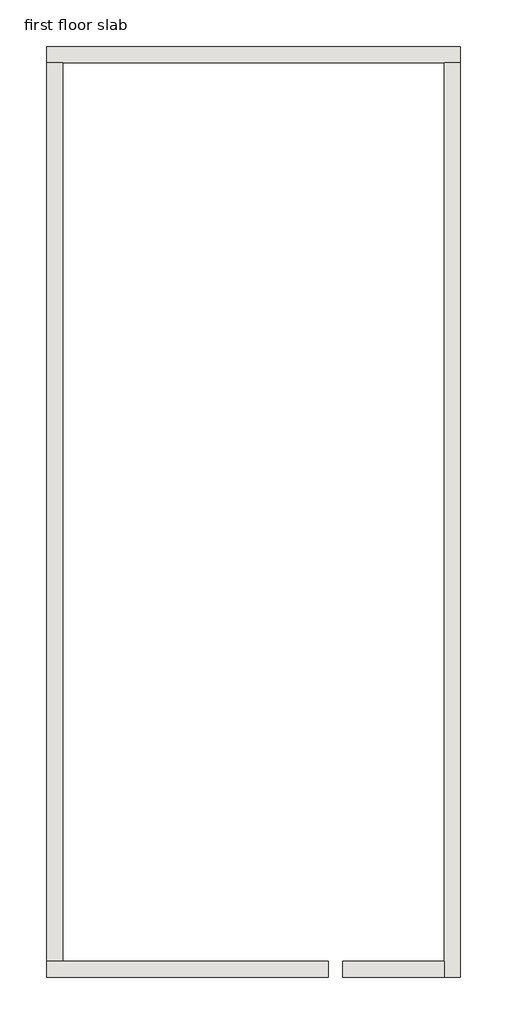
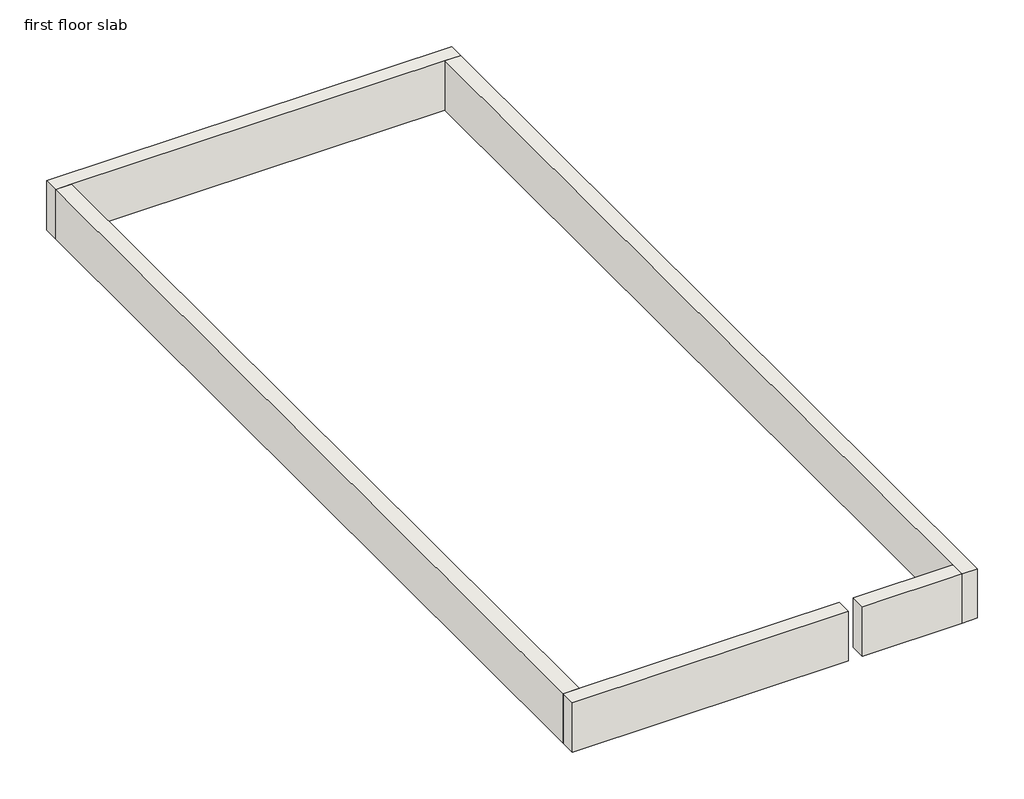
# One storey: 5 walls.
"""IFC4 building model written with IfcOpenShell, lengths in millimetres."""

from ifc_helpers import new_model, si_unit, frame, origin, place, context, project, spatial, polyline, outline, extrude, faceted_brep, element, save

model = new_model("IFC4")

# Units and contexts
model_context = context("Model", 3, world=origin())
ifc_project = project(units=[si_unit("LENGTHUNIT", "METRE", prefix="MILLI")], contexts=[model_context])

# Site, building, storey
site = spatial("IfcSite", under=ifc_project)
building = spatial("IfcBuilding", under=site)
storey = spatial("IfcBuildingStorey", under=building, Name="first floor slab", Elevation=6705.6)

# Walls
placement = place(None, origin())
element("IfcWall", 1, ObjectType="wall 9\"", at=placement, inside=storey, context=model_context, shape_type="Brep", body=[
    faceted_brep([(-12403.8986863, -3151.661407, 6705.6), (-16197.9371373, -3151.661407, 6705.6), (-16426.5371373, -3151.661407, 6705.6), (-16426.5371373, -3151.661407, 7467.6), (-16197.9371373, -3151.661407, 7467.6), (-12403.8986863, -3151.661407, 7467.6), (-12403.8986863, -3380.261407, 6705.6), (-12403.8986863, -3380.261407, 7467.6), (-16426.5371373, -3380.261407, 7467.6), (-16426.5371373, -3380.261407, 6705.6)], [[[0, 1, 2, 3, 4, 5]], [[6, 7, 8, 9]], [[2, 1, 0, 6, 9]], [[5, 4, 3, 8, 7]], [[0, 5, 7, 6]], [[3, 2, 9, 8]]]),
])
element("IfcWall", 2, ObjectType="wall 9\"", at=placement, inside=storey, context=model_context, shape_type="Brep", body=[
    faceted_brep([(-16426.5371373, 9675.338593, 6705.6), (-16197.9371373, 9675.338593, 6705.6), (-10749.6371373, 9675.338593, 6705.6), (-10521.0371373, 9675.338593, 6705.6), (-10521.0371373, 9675.338593, 7467.6), (-10749.6371373, 9675.338593, 7467.6), (-16197.9371373, 9675.338593, 7467.6), (-16426.5371373, 9675.338593, 7467.6), (-16426.5371373, 9903.938593, 6705.6), (-16426.5371373, 9903.938593, 7467.6), (-10521.0371373, 9903.938593, 7467.6), (-10521.0371373, 9903.938593, 6705.6)], [[[0, 1, 2, 3, 4, 5, 6, 7]], [[8, 9, 10, 11]], [[3, 2, 1, 0, 8, 11]], [[7, 6, 5, 4, 10, 9]], [[4, 3, 11, 10]], [[0, 7, 9, 8]]]),
])
element("IfcWall", 3, ObjectType="wall 9\"", at=placement, inside=storey, context=model_context, shape_type="Brep", body=[
    faceted_brep([(-10749.6371373, 9675.338593, 6705.6), (-10749.6371373, -3151.661407, 6705.6), (-10749.6371373, -3380.261407, 6705.6), (-10749.6371373, -3380.261407, 7467.6), (-10749.6371373, -3151.661407, 7467.6), (-10749.6371373, 9675.338593, 7467.6), (-10521.0371373, 9675.338593, 6705.6), (-10521.0371373, 9675.338593, 7467.6), (-10521.0371373, -3380.261407, 7467.6), (-10521.0371373, -3380.261407, 6705.6)], [[[0, 1, 2, 3, 4, 5]], [[6, 7, 8, 9]], [[2, 1, 0, 6, 9]], [[5, 4, 3, 8, 7]], [[0, 5, 7, 6]], [[3, 2, 9, 8]]]),
])
element("IfcWall", 4, ObjectType="wall 9\"", at=placement, inside=storey, context=model_context, shape_type="SweptSolid", body=[
    extrude(outline(polyline([(-12197.4371373, -3151.661407), (-10749.6371373, -3151.661407), (-10749.6371373, -3380.261407), (-12197.4371373, -3380.261407), (-12197.4371373, -3151.661407)])), frame((0.0, 0.0, 6705.6), z_axis=(0.0, 0.0, 1.0), x_axis=(1.0, 0.0, 0.0)), (0.0, 0.0, 1.0), 762.0),
])
element("IfcWall", 5, ObjectType="wall 9\"", at=placement, inside=storey, context=model_context, shape_type="SweptSolid", body=[
    extrude(outline(polyline([(-16197.9371373, 9675.338593), (-16197.9371373, -3151.661407), (-16426.5371373, -3151.661407), (-16426.5371373, 9675.338593), (-16197.9371373, 9675.338593)])), frame((0.0, 0.0, 6705.6), z_axis=(0.0, 0.0, 1.0), x_axis=(1.0, 0.0, 0.0)), (0.0, 0.0, 1.0), 762.0),
])

save(model, "model.ifc")

# Revit data of these elements
# Type "wall 9\""
#   Assembly Code = "B2010"
#   Layers, outside or top first: 0' - 9" no material (function 1)
# Element 1 (IfcWall, "wall 9\"")
#   Top Offset = 0' - 0"
#   Base Offset = 0' - 0"
#   wall height = 2' - 6"
#   Phase Created = New Construction
#   Base Constraint = first floor slab
#   Top Constraint = level 4
#   Materials on its faces: "1. WALL PAINT", "Default Wall"
# Elements 2, 5 (IfcWall, "wall 9\"")
#   Top Offset = 0' - 0"
#   Base Offset = 0' - 0"
#   Unconnected Height = 2' - 6"
#   wall height = 2' - 6"
#   Phase Created = New Construction
#   Base Constraint = first floor slab
#   Materials on its faces: "1. WALL PAINT", "Default Wall"
# Elements 3, 4 (IfcWall, "wall 9\"")
#   Top Offset = 0' - 0"
#   Base Offset = 0' - 0"
#   Unconnected Height = 2' - 6"
#   wall height = 2' - 6"
#   Phase Created = New Construction
#   Base Constraint = first floor slab
#   Materials on its faces: "Default Wall", "1. WALL PAINT"
# Materials
#   "1. WALL PAINT": class "Generic", colour RGB 120 120 120, transparency 0, Cost = 0
#   "Default Wall": colour RGB 128 128 128, transparency 0, Cost = 0
